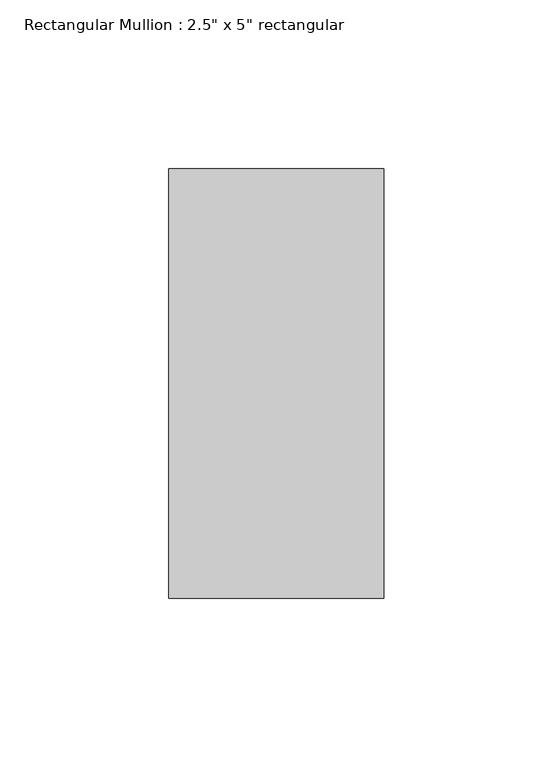
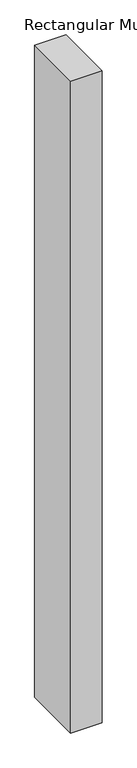
"""IFC4 building model written with IfcOpenShell, lengths in millimetres: member geometry."""

from ifc_helpers import new_model, si_unit, frame, origin, place, context, project, spatial, polyline, outline, extrude, source, transform, mapped, element, save


def member_a4baedd8(model_context):
    return source(origin(), model_context, "Body", "SweptSolid", [
        extrude(outline(polyline([(0.0, 63.5), (0.0, -63.5), (-63.5, -63.5), (-63.5, 63.5), (0.0, 63.5)])), frame((0.0, 0.0, -1403.3499998), z_axis=(0.0, 0.0, 1.0), x_axis=(1.0, 0.0, 0.0)), (0.0, 0.0, 1.0), 1403.3499998),
    ])


if __name__ == "__main__":
    model = new_model("IFC4")
    model_context = context("Model", 3, world=origin())
    ifc_project = project(units=[si_unit("LENGTHUNIT", "METRE", prefix="MILLI")], contexts=[model_context])
    site = spatial("IfcSite", under=ifc_project)
    building = spatial("IfcBuilding", under=site)
    placement = place(None, origin())
    member_shape = member_a4baedd8(model_context)
    element("IfcMember", 1, ObjectType="Rectangular Mullion : 2.5\" x 5\" rectangular", at=placement, inside=building, context=model_context, shape_type="MappedRepresentation", body=[
        mapped(member_shape, transform((0.0, 0.0, 0.0), x_axis=(1.0, 0.0, 0.0), y_axis=(0.0, 1.0, 0.0), z_axis=(0.0, 0.0, 1.0))),
    ])
    save(model, "model.ifc")

# Revit data of these elements
# Type "Rectangular Mullion : 2.5\" x 5\" rectangular"
#   built-in parameter 1007304 = 0.416667 (stored number, unit not read)
#   built-in parameter 1007301 = 0.104167 (stored number, unit not read)
#   built-in parameter 1007300 = 0.104167 (stored number, unit not read)
# Element 1 (IfcMember, "Rectangular Mullion : 2.5\" x 5\" rectangular")
#   Materials on its faces: "metal black"
# Materials
#   "metal black": class "Generic", colour RGB 120 120 120, transparency 0, Cost = 0
